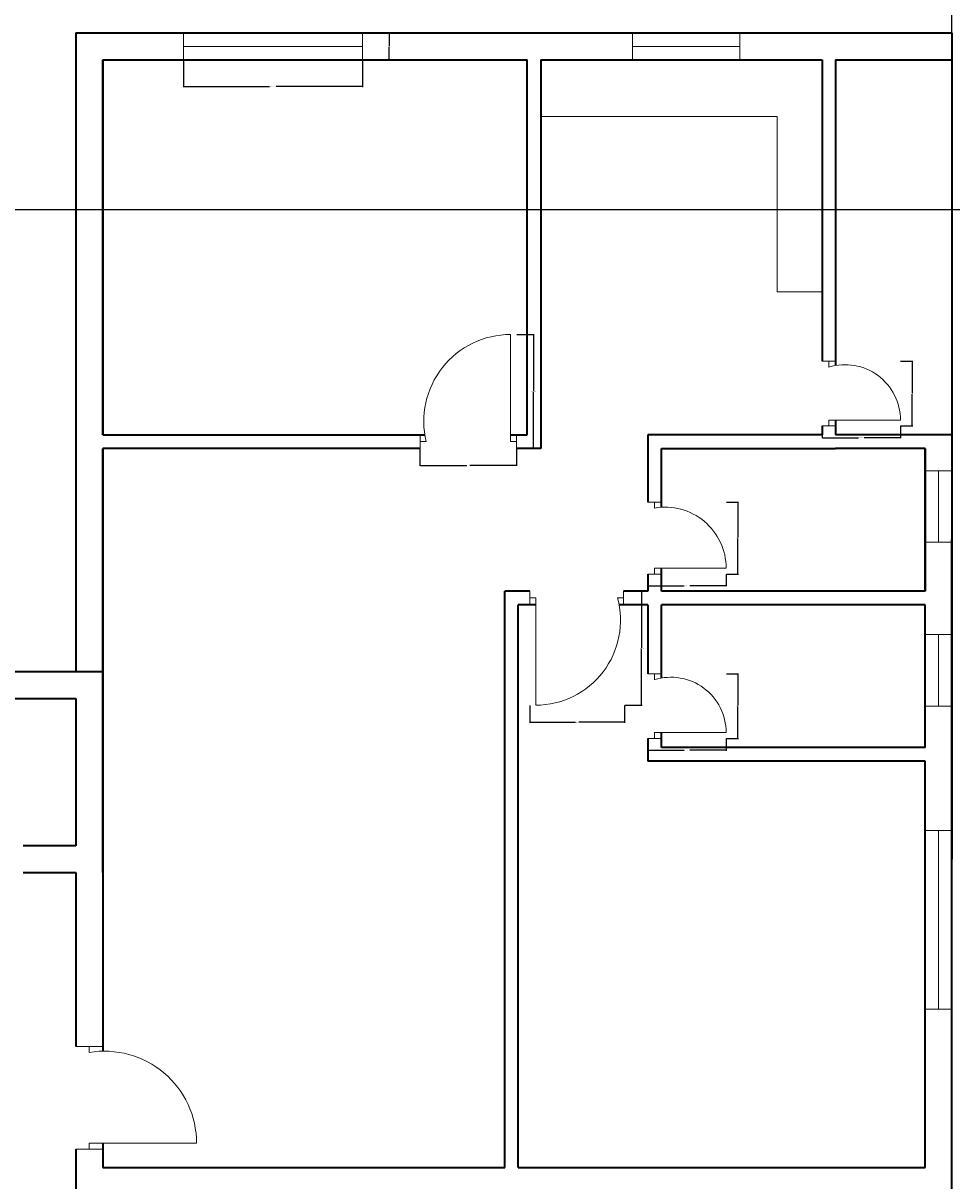
# Model space of a CAD drawing. Units: inches. Extents: x 2120 to 4013, y 1390 to 3019.
# Tile 53 of 59: x 3507 to 3819, y 1967 to 2356. Entities that reach past the tile are written whole.
import ezdxf

# ---------------------------------------------------------------- set-up
doc = ezdxf.new("R2010")
doc.units = ezdxf.units.IN
for name, color, linetype, lineweight in [('A-ANNO-DIMS', 2, 'Continuous', 18), ('A-ANNO-SYMB', 2, 'Continuous', 25), ('A-DOOR', 3, 'Continuous', 18), ('A-FLOR-CASE', 8, 'Continuous', 18), ('A-FURN', 8, 'Continuous', 13), ('A-GLAZ', 4, 'Continuous', 18), ('A-WALL', 7, 'Continuous', 35)]:
    doc.layers.add(name, color=color, linetype=linetype, lineweight=lineweight)
doc.styles.get("Standard").update_dxf_attribs({"font": 'arial.ttf'})
doc.dimstyles.get("Standard").update_dxf_attribs({"dimtxt": 0.18, "dimasz": 0.18, "dimexe": 0.18, "dimexo": 0.0625, "dimgap": 0.09, "dimtad": 0, "dimtih": 1, "dimtoh": 1, "dimdec": 4, "dimzin": 0, "dimdsep": 46, "dimtxsty": 'Standard', "dimcen": 0.09, "dimadec": 0, "dimazin": 0, "dimtfac": 1, "dimtdec": 4, "dimtofl": 0, "dimtmove": 0, "dimatfit": 3, "dimfxl": 1, "dimtolj": 1, "dimtzin": 0, "dimarcsym": 0})

# ---------------------------------------------------------------- blocks, each defined once
blk = doc.blocks.new('DOOR-SWING-24IN-106p92DEG')
for p, q in [((4.5, 21.79), (0, 21.79)), ((0, 21.79), (2.25, 21.79)), ((2.25, 21.79), (2.25, 19.79)), ((2.25, 0), (2.25, 2)), ((2.25, 2), (26.25, 2)), ((0, 0), (4.5, 0)), ((4.5, 0), (2.25, 0))]:
    blk.add_line(p, q)
blk.add_arc((7.66, 2), 18.59, 0, 106.9181)
blk = doc.blocks.new('DOOR-SWING-24IN-99p98DEG')
for p, q in [((0, 24.15), (4.5, 24.15)), ((4.5, 24.15), (2.25, 24.15)), ((2.25, 24.15), (2.25, 22.15)), ((4.5, 0), (0, 0)), ((0, 0), (2.25, 0)), ((2.25, 0), (2.25, 2)), ((2.25, 2), (26.25, 2))]:
    blk.add_line(p, q)
blk.add_arc((5.79, 2), 20.46, 0, 99.9792)
blk = doc.blocks.new('DOOR-SWING-24IN-107p06DEG')
for p, q in [((0, 21.74), (4.5, 21.74)), ((4.5, 21.74), (2.25, 21.74)), ((2.25, 21.74), (2.25, 19.74)), ((4.5, 0), (0, 0)), ((0, 0), (0, 0)), ((0, 0), (2.25, 0)), ((2.25, 0), (2.25, 2)), ((2.25, 2), (26.25, 2))]:
    blk.add_line(p, q)
blk.add_arc((7.69, 2), 18.56, 0, 107.0611)
blk = doc.blocks.new('DOOR-SWING-36IN-103p63DEG')
for p, q in [((30.32, 2.25), (30.32, 38.25)), ((0, 4.5), (0, 0)), ((32.32, 4.5), (32.32, 0)), ((0, 0), (0, 2.25)), ((0, 2.25), (2, 2.25)), ((32.32, 2.25), (30.32, 2.25)), ((32.32, 0), (32.32, 2.25))]:
    blk.add_line(p, q)
blk.add_arc((30.32, 9.11), 29.14, 90, 193.6269)
blk = doc.blocks.new('DOOR-SWING-36IN-105p32DEG')
for p, q in [((0, 33.75), (0, 38.25)), ((0, 38.25), (0, 36)), ((0, 36), (2, 36)), ((2, 36), (2, 0)), ((31.46, 36), (29.46, 36)), ((31.46, 33.75), (31.46, 38.25)), ((31.46, 38.25), (31.46, 36))]:
    blk.add_line(p, q)
blk.add_arc((2, 28.48), 28.48, 270, 15.3194)
blk = doc.blocks.new('WIN-PLAN-24IN-02')
for p, q in [((0, 0), (0, 9)), ((0, 9), (0, 4.5)), ((24, 4.5), (24, 9)), ((24, 9), (24, 0)), ((0, 4.5), (24, 4.5))]:
    blk.add_line(p, q)
blk = doc.blocks.new('WIN-PLAN-24IN-04')
for p, q in [((0, 24), (9, 24)), ((9, 24), (4.5, 24)), ((4.5, 24), (4.5, 0)), ((9, 24), (9, 24)), ((4.5, 0), (0, 0)), ((0, 0), (9, 0))]:
    blk.add_line(p, q)
blk = doc.blocks.new('WIN-PLAN-60IN')
for p, q in [((0, 9), (0, 0)), ((60, 4.5), (60, 9)), ((60, 9), (60, 0)), ((0, 0), (0, 4.5)), ((0, 4.5), (60, 4.5))]:
    blk.add_line(p, q)
blk = doc.blocks.new('WIN-PLAN-60IN-02')
for p, q in [((0, 0), (0, 9)), ((0, 9), (0, 4.5)), ((60, 4.5), (60, 9)), ((60, 9), (60, 0)), ((0, 4.5), (60, 4.5))]:
    blk.add_line(p, q)
blk = doc.blocks.new('WIN-PLAN-36IN')
for p, q in [((0, 0), (0, 9)), ((0, 9), (0, 4.5)), ((36, 4.5), (36, 9)), ((36, 9), (36, 0)), ((0, 4.5), (36, 4.5))]:
    blk.add_line(p, q)
blk = doc.blocks.new('*D121')
at = {"layer": 'A-ANNO-DIMS', "color": 0, "lineweight": -2, "transparency": 16777216}
for p, q in [((3775.23, 2220.48), (3775.23, 2216.43)), ((3801.48, 2220.48), (3801.48, 2216.43)), ((3775.41, 2216.61), (3787.37, 2216.61)), ((3801.3, 2216.61), (3789.35, 2216.61))]:
    blk.add_line(p, q, dxfattribs=at)
at = {"layer": 'A-ANNO-DIMS', "color": 0, "transparency": 16777216}
for points in [[(3775.41, 2216.64), (3775.41, 2216.58), (3775.23, 2216.61)], [(3801.3, 2216.64), (3801.3, 2216.58), (3801.48, 2216.61)]]:
    blk.add_solid(points, dxfattribs=at)
at = {"layer": 'Defpoints', "color": 0, "transparency": 16777216}
for p in [(3775.23, 2220.54), (3801.48, 2220.54), (3801.48, 2216.61)]:
    blk.add_point(p, dxfattribs=at)
at = {"layer": 'A-ANNO-DIMS', "color": 0, "transparency": 16777216, "insert": (3788.36, 2216.61), "char_height": 0.18, "attachment_point": 5}
blk.add_mtext('\\A1;SWING 26 TYP.', dxfattribs=at)
blk = doc.blocks.new('*D122')
at = {"layer": 'A-ANNO-DIMS', "color": 0, "lineweight": -2, "transparency": 16777216}
for p, q in [((3801.55, 2242.33), (3805.6, 2242.33)), ((3805.42, 2242.15), (3805.42, 2231.62)), ((3805.42, 2220.72), (3805.42, 2231.25)), ((3801.55, 2220.54), (3805.6, 2220.54))]:
    blk.add_line(p, q, dxfattribs=at)
at = {"layer": 'A-ANNO-DIMS', "color": 0, "transparency": 16777216}
for points in [[(3805.39, 2242.15), (3805.45, 2242.15), (3805.42, 2242.33)], [(3805.39, 2220.72), (3805.45, 2220.72), (3805.42, 2220.54)]]:
    blk.add_solid(points, dxfattribs=at)
at = {"layer": 'Defpoints', "color": 0, "transparency": 16777216}
for p in [(3801.48, 2242.33), (3805.42, 2242.33), (3801.48, 2220.54)]:
    blk.add_point(p, dxfattribs=at)
at = {"layer": 'A-ANNO-DIMS', "color": 0, "transparency": 16777216, "insert": (3805.42, 2231.44), "char_height": 0.18, "attachment_point": 5}
blk.add_mtext('\\A1;22 TYP.', dxfattribs=at)
blk = doc.blocks.new('*D123')
at = {"layer": 'A-ANNO-DIMS', "color": 0, "lineweight": -2, "transparency": 16777216}
for p, q in [((3716.73, 2170.76), (3716.73, 2166.7)), ((3742.98, 2170.76), (3742.98, 2166.7)), ((3716.91, 2166.88), (3728.87, 2166.88)), ((3742.8, 2166.88), (3730.85, 2166.88))]:
    blk.add_line(p, q, dxfattribs=at)
at = {"layer": 'A-ANNO-DIMS', "color": 0, "transparency": 16777216}
for points in [[(3716.91, 2166.91), (3716.91, 2166.85), (3716.73, 2166.88)], [(3742.8, 2166.91), (3742.8, 2166.85), (3742.98, 2166.88)]]:
    blk.add_solid(points, dxfattribs=at)
at = {"layer": 'Defpoints', "color": 0, "transparency": 16777216}
for p in [(3716.73, 2170.82), (3742.98, 2170.82), (3742.98, 2166.88)]:
    blk.add_point(p, dxfattribs=at)
at = {"layer": 'A-ANNO-DIMS', "color": 0, "transparency": 16777216, "insert": (3729.86, 2166.88), "char_height": 0.18, "attachment_point": 5}
blk.add_mtext('\\A1;SWING 26 TYP.', dxfattribs=at)
blk = doc.blocks.new('*D124')
at = {"layer": 'A-ANNO-DIMS', "color": 0, "lineweight": -2, "transparency": 16777216}
for p, q in [((3743.05, 2194.97), (3747.1, 2194.97)), ((3746.92, 2194.79), (3746.92, 2183.07)), ((3746.92, 2171), (3746.92, 2182.71)), ((3743.05, 2170.82), (3747.1, 2170.82))]:
    blk.add_line(p, q, dxfattribs=at)
at = {"layer": 'A-ANNO-DIMS', "color": 0, "transparency": 16777216}
for points in [[(3746.89, 2194.79), (3746.95, 2194.79), (3746.92, 2194.97)], [(3746.89, 2171), (3746.95, 2171), (3746.92, 2170.82)]]:
    blk.add_solid(points, dxfattribs=at)
at = {"layer": 'Defpoints', "color": 0, "transparency": 16777216}
for p in [(3742.98, 2194.97), (3746.92, 2194.97), (3742.98, 2170.82)]:
    blk.add_point(p, dxfattribs=at)
at = {"layer": 'A-ANNO-DIMS', "color": 0, "transparency": 16777216, "insert": (3746.92, 2182.89), "char_height": 0.18, "attachment_point": 5}
blk.add_mtext('\\A1;24 TYP.', dxfattribs=at)
blk = doc.blocks.new('*D125')
at = {"layer": 'A-ANNO-DIMS', "color": 0, "lineweight": -2, "transparency": 16777216}
for p, q in [((3716.73, 2115.54), (3716.73, 2111.49)), ((3742.98, 2115.54), (3742.98, 2111.49)), ((3716.91, 2111.67), (3728.87, 2111.67)), ((3742.8, 2111.67), (3730.85, 2111.67))]:
    blk.add_line(p, q, dxfattribs=at)
at = {"layer": 'A-ANNO-DIMS', "color": 0, "transparency": 16777216}
for points in [[(3716.91, 2111.7), (3716.91, 2111.64), (3716.73, 2111.67)], [(3742.8, 2111.7), (3742.8, 2111.64), (3742.98, 2111.67)]]:
    blk.add_solid(points, dxfattribs=at)
at = {"layer": 'Defpoints', "color": 0, "transparency": 16777216}
for p in [(3716.73, 2115.6), (3742.98, 2115.6), (3742.98, 2111.67)]:
    blk.add_point(p, dxfattribs=at)
at = {"layer": 'A-ANNO-DIMS', "color": 0, "transparency": 16777216, "insert": (3729.86, 2111.67), "char_height": 0.18, "attachment_point": 5}
blk.add_mtext('\\A1;SWING 26 TYP.', dxfattribs=at)
blk = doc.blocks.new('*D126')
at = {"layer": 'A-ANNO-DIMS', "color": 0, "lineweight": -2, "transparency": 16777216}
for p, q in [((3743.05, 2137.34), (3747.1, 2137.34)), ((3746.92, 2137.16), (3746.92, 2126.65)), ((3746.92, 2115.78), (3746.92, 2126.29)), ((3743.05, 2115.6), (3747.1, 2115.6))]:
    blk.add_line(p, q, dxfattribs=at)
at = {"layer": 'A-ANNO-DIMS', "color": 0, "transparency": 16777216}
for points in [[(3746.89, 2137.16), (3746.95, 2137.16), (3746.92, 2137.34)], [(3746.89, 2115.78), (3746.95, 2115.78), (3746.92, 2115.6)]]:
    blk.add_solid(points, dxfattribs=at)
at = {"layer": 'Defpoints', "color": 0, "transparency": 16777216}
for p in [(3742.98, 2137.34), (3746.92, 2137.34), (3742.98, 2115.6)]:
    blk.add_point(p, dxfattribs=at)
at = {"layer": 'A-ANNO-DIMS', "color": 0, "transparency": 16777216, "insert": (3746.92, 2126.47), "char_height": 0.18, "attachment_point": 5}
blk.add_mtext('\\A1;22 TYP.', dxfattribs=at)
blk = doc.blocks.new('*D151')
at = {"layer": 'A-ANNO-DIMS', "color": 0, "lineweight": -2, "transparency": 16777216}
for p, q in [((3672.7, 2251.28), (3678.56, 2251.28)), ((3678.38, 2251.1), (3678.38, 2232.34)), ((3678.38, 2213.21), (3678.38, 2231.97)), ((3672.7, 2213.03), (3678.56, 2213.03))]:
    blk.add_line(p, q, dxfattribs=at)
at = {"layer": 'A-ANNO-DIMS', "color": 0, "transparency": 16777216}
for points in [[(3678.35, 2251.1), (3678.41, 2251.1), (3678.38, 2251.28)], [(3678.35, 2213.21), (3678.41, 2213.21), (3678.38, 2213.03)]]:
    blk.add_solid(points, dxfattribs=at)
at = {"layer": 'Defpoints', "color": 0, "transparency": 16777216}
for p in [(3672.64, 2251.28), (3678.38, 2251.28), (3672.64, 2213.03)]:
    blk.add_point(p, dxfattribs=at)
at = {"layer": 'A-ANNO-DIMS', "color": 0, "transparency": 16777216, "insert": (3678.38, 2232.16), "char_height": 0.18, "attachment_point": 5}
blk.add_mtext('\\A1;SWING 38 TYP.', dxfattribs=at)
blk = doc.blocks.new('*D152')
at = {"layer": 'A-ANNO-DIMS', "color": 0, "lineweight": -2, "transparency": 16777216}
for p, q in [((3640.22, 2212.97), (3640.22, 2207.11)), ((3672.64, 2212.97), (3672.64, 2207.11)), ((3640.4, 2207.29), (3655.9, 2207.29)), ((3672.46, 2207.29), (3656.96, 2207.29))]:
    blk.add_line(p, q, dxfattribs=at)
at = {"layer": 'A-ANNO-DIMS', "color": 0, "transparency": 16777216}
for points in [[(3640.4, 2207.32), (3640.4, 2207.26), (3640.22, 2207.29)], [(3672.46, 2207.32), (3672.46, 2207.26), (3672.64, 2207.29)]]:
    blk.add_solid(points, dxfattribs=at)
at = {"layer": 'Defpoints', "color": 0, "transparency": 16777216}
for p in [(3640.22, 2213.03), (3672.64, 2213.03), (3672.64, 2207.29)]:
    blk.add_point(p, dxfattribs=at)
at = {"layer": 'A-ANNO-DIMS', "color": 0, "transparency": 16777216, "insert": (3656.43, 2207.29), "char_height": 0.18, "attachment_point": 5}
blk.add_mtext('\\A1;32 TYP.', dxfattribs=at)
blk = doc.blocks.new('*D153')
at = {"layer": 'A-ANNO-DIMS', "color": 0, "lineweight": -2, "transparency": 16777216}
for p, q in [((3708.93, 2165.03), (3714.78, 2165.03)), ((3714.6, 2164.85), (3714.6, 2146.09)), ((3714.6, 2126.96), (3714.6, 2145.72)), ((3708.93, 2126.78), (3714.78, 2126.78))]:
    blk.add_line(p, q, dxfattribs=at)
at = {"layer": 'A-ANNO-DIMS', "color": 0, "transparency": 16777216}
for points in [[(3714.57, 2164.85), (3714.63, 2164.85), (3714.6, 2165.03)], [(3714.57, 2126.96), (3714.63, 2126.96), (3714.6, 2126.78)]]:
    blk.add_solid(points, dxfattribs=at)
at = {"layer": 'Defpoints', "color": 0, "transparency": 16777216}
for p in [(3708.86, 2165.03), (3714.6, 2165.03), (3708.86, 2126.78)]:
    blk.add_point(p, dxfattribs=at)
at = {"layer": 'A-ANNO-DIMS', "color": 0, "transparency": 16777216, "insert": (3714.6, 2145.91), "char_height": 0.18, "attachment_point": 5}
blk.add_mtext('\\A1;SWING 38 TYP.', dxfattribs=at)
blk = doc.blocks.new('*D154')
at = {"layer": 'A-ANNO-DIMS', "color": 0, "lineweight": -2, "transparency": 16777216}
for p, q in [((3677.05, 2126.72), (3677.05, 2120.86)), ((3708.86, 2126.72), (3708.86, 2120.86)), ((3677.23, 2121.04), (3692.43, 2121.04)), ((3708.68, 2121.04), (3693.49, 2121.04))]:
    blk.add_line(p, q, dxfattribs=at)
at = {"layer": 'A-ANNO-DIMS', "color": 0, "transparency": 16777216}
for points in [[(3677.23, 2121.07), (3677.23, 2121.01), (3677.05, 2121.04)], [(3708.68, 2121.07), (3708.68, 2121.01), (3708.86, 2121.04)]]:
    blk.add_solid(points, dxfattribs=at)
at = {"layer": 'Defpoints', "color": 0, "transparency": 16777216}
for p in [(3677.05, 2126.78), (3708.86, 2126.78), (3708.86, 2121.04)]:
    blk.add_point(p, dxfattribs=at)
at = {"layer": 'A-ANNO-DIMS', "color": 0, "transparency": 16777216, "insert": (3692.96, 2121.04), "char_height": 0.18, "attachment_point": 5}
blk.add_mtext('\\A1;32 TYP.', dxfattribs=at)
blk = doc.blocks.new('*D173')
at = {"layer": 'A-ANNO-DIMS', "color": 0, "lineweight": -2, "transparency": 16777216}
for p, q in [((3560.88, 2343.47), (3560.88, 2334.35)), ((3620.88, 2343.47), (3620.88, 2334.35)), ((3561.06, 2334.53), (3589.76, 2334.53)), ((3620.7, 2334.53), (3592, 2334.53))]:
    blk.add_line(p, q, dxfattribs=at)
at = {"layer": 'A-ANNO-DIMS', "color": 0, "transparency": 16777216}
for points in [[(3561.06, 2334.56), (3561.06, 2334.5), (3560.88, 2334.53)], [(3620.7, 2334.56), (3620.7, 2334.5), (3620.88, 2334.53)]]:
    blk.add_solid(points, dxfattribs=at)
at = {"layer": 'Defpoints', "color": 0, "transparency": 16777216}
for p in [(3560.88, 2343.53), (3620.88, 2343.53), (3620.88, 2334.53)]:
    blk.add_point(p, dxfattribs=at)
at = {"layer": 'A-ANNO-DIMS', "color": 0, "transparency": 16777216, "insert": (3590.88, 2334.53), "char_height": 0.18, "attachment_point": 5}
blk.add_mtext('\\A1;WINDOW 60 TYP.', dxfattribs=at)
blk = doc.blocks.new('*D174')
at = {"layer": 'A-ANNO-DIMS', "color": 0, "lineweight": -2, "transparency": 16777216}
for p, q in [((3620.94, 2352.53), (3630.06, 2352.53)), ((3629.88, 2352.35), (3629.88, 2348.21)), ((3629.88, 2343.71), (3629.88, 2347.85)), ((3620.94, 2343.53), (3630.06, 2343.53))]:
    blk.add_line(p, q, dxfattribs=at)
at = {"layer": 'A-ANNO-DIMS', "color": 0, "transparency": 16777216}
for points in [[(3629.85, 2352.35), (3629.91, 2352.35), (3629.88, 2352.53)], [(3629.85, 2343.71), (3629.91, 2343.71), (3629.88, 2343.53)]]:
    blk.add_solid(points, dxfattribs=at)
at = {"layer": 'Defpoints', "color": 0, "transparency": 16777216}
for p in [(3620.88, 2352.53), (3629.88, 2352.53), (3620.88, 2343.53)]:
    blk.add_point(p, dxfattribs=at)
at = {"layer": 'A-ANNO-DIMS', "color": 0, "transparency": 16777216, "insert": (3629.88, 2348.03), "char_height": 0.18, "attachment_point": 5}
blk.add_mtext('\\A1;9 TYP.', dxfattribs=at)
blk = doc.blocks.new('*D216')
at = {"layer": 'A-ANNO-DIMS', "color": 0, "lineweight": -2, "transparency": 16777216}
for p, q in [((3071.73, 2352.59), (3071.73, 2396.46)), ((3071.91, 2396.28), (3444.95, 2396.28)), ((3818.55, 2396.28), (3445.52, 2396.28)), ((3818.73, 2352.59), (3818.73, 2396.46))]:
    blk.add_line(p, q, dxfattribs=at)
at = {"layer": 'A-ANNO-DIMS', "color": 0, "transparency": 16777216}
for points in [[(3071.91, 2396.31), (3071.91, 2396.25), (3071.73, 2396.28)], [(3818.55, 2396.31), (3818.55, 2396.25), (3818.73, 2396.28)]]:
    blk.add_solid(points, dxfattribs=at)
at = {"layer": 'Defpoints', "color": 0, "transparency": 16777216}
for p in [(3818.73, 2396.28), (3071.73, 2352.53), (3818.73, 2352.53)]:
    blk.add_point(p, dxfattribs=at)
at = {"layer": 'A-ANNO-DIMS', "color": 0, "transparency": 16777216, "insert": (3445.23, 2396.28), "char_height": 0.18, "attachment_point": 5}
blk.add_mtext('\\A1;747', dxfattribs=at)

msp = doc.modelspace()

# ---------------------------------------------------------------- linework, layer by layer
at = {"layer": 'A-ANNO-SYMB'}
msp.add_line((3024.2377, 2293.2324), (3883.8033, 2293.2324), dxfattribs=at)
at = {"layer": 'A-DOOR'}
for p, q in [((3533.7347, 2012.1531), (3524.7347, 2012.1531)), ((3529.2347, 2012.1531), (3529.2347, 2010.1531)), ((3529.2347, 1977.7015), (3529.2347, 1979.7015)), ((3529.2347, 1979.7015), (3565.2347, 1979.7015)), ((3533.7347, 1977.7015), (3524.7347, 1977.7015)), ((3524.7347, 1977.7015), (3529.2347, 1977.7015))]:
    msp.add_line(p, q, dxfattribs=at)
msp.add_arc((3534.3555, 1979.7015), 30.8792, 360, 99.545687, dxfattribs=at)
at = {"layer": 'A-FLOR-CASE'}
for p, q in [((3680.7347, 2324.4835), (3760.0811, 2324.4835)), ((3760.0811, 2324.4835), (3760.0811, 2265.6008)), ((3760.0811, 2265.6008), (3775.2347, 2265.6008))]:
    msp.add_line(p, q, dxfattribs=at)
at = {"layer": 'A-FURN'}
for p, q in [((3558.231, 2343.531), (3606.0213, 2343.531)), ((3809.7347, 2054.2058), (3809.7347, 2006.4156))]:
    msp.add_line(p, q, dxfattribs=at)
at = {"layer": 'A-WALL'}
for p, q in [((3524.7347, 2352.531), (3818.7347, 2352.531)), ((3524.7347, 2352.531), (3524.7347, 2138.031)), ((3818.7347, 2352.531), (3818.7347, 2075.031)), ((3533.7347, 2343.531), (3676.2347, 2343.531)), ((3533.7347, 2217.531), (3533.7347, 2343.531)), ((3533.7347, 2343.531), (3533.7347, 2217.531)), ((3676.2347, 2217.531), (3676.2347, 2343.531)), ((3680.7347, 2343.531), (3775.2347, 2343.531)), ((3680.7347, 2343.531), (3680.7347, 2217.531)), ((3775.2347, 2343.531), (3775.2347, 2242.3281)), ((3779.7347, 2343.531), (3818.7347, 2343.531)), ((3779.7347, 2343.531), (3779.7347, 2240.8622)), ((3779.7347, 2343.531), (3818.7347, 2343.531)), ((3775.2347, 2220.5425), (3775.2347, 2217.531)), ((3779.7347, 2222.5425), (3779.7347, 2217.531)), ((3533.7347, 2217.531), (3641.87, 2217.531)), ((3670.6379, 2217.531), (3676.2347, 2217.531)), ((3680.7347, 2217.531), (3680.7347, 2213.031)), ((3720.7767, 2217.531), (3716.7347, 2217.531)), ((3716.7347, 2217.531), (3716.7347, 2213.031)), ((3775.2347, 2217.531), (3720.7767, 2217.531)), ((3818.7347, 2217.531), (3779.7347, 2217.531)), ((3533.7347, 2138.031), (3533.7347, 2213.031)), ((3640.3224, 2213.031), (3533.7347, 2213.031)), ((3533.7347, 2213.031), (3533.7347, 2010.5745)), ((3680.7347, 2213.031), (3672.6379, 2213.031)), ((3716.7347, 2213.031), (3716.7347, 2194.9663)), ((3721.2347, 2213.031), (3779.7347, 2213.031)), ((3721.2347, 2193.2348), (3721.2347, 2213.031)), ((3809.7347, 2213.031), (3779.7347, 2213.031)), ((3809.7347, 2182.408), (3809.7347, 2213.031)), ((3809.7347, 2213.031), (3809.7347, 2165.031)), ((3809.7347, 2165.031), (3809.7347, 2182.408)), ((3818.7347, 1971.531), (3818.7347, 2182.408)), ((3716.7347, 2170.8205), (3716.7347, 2165.031)), ((3721.2347, 2165.031), (3721.2347, 2172.8205)), ((3668.7347, 1971.531), (3668.7347, 2165.031)), ((3677.0538, 2165.031), (3668.7347, 2165.031)), ((3716.7347, 2165.031), (3708.5184, 2165.031)), ((3809.7347, 2165.031), (3721.2347, 2165.031)), ((3673.2347, 1971.531), (3673.2347, 2160.531)), ((3679.0538, 2160.531), (3673.2347, 2160.531)), ((3716.7347, 2160.531), (3707.0377, 2160.531)), ((3716.7347, 2160.531), (3716.7347, 2137.3432)), ((3809.7347, 2160.531), (3721.2347, 2160.531)), ((3721.2347, 2135.8828), (3721.2347, 2160.531)), ((3809.7347, 2112.531), (3809.7347, 2160.531)), ((3533.7347, 2138.031), (3437.7347, 2138.031)), ((3533.7347, 2129.031), (3533.7347, 2138.031)), ((3446.7347, 2129.031), (3524.7347, 2129.031)), ((3524.7347, 2129.031), (3524.7347, 2079.531)), ((3533.7347, 2070.531), (3533.7347, 2129.031)), ((3716.7347, 2115.6039), (3716.7347, 2108.031)), ((3721.2347, 2112.531), (3721.2347, 2117.6039)), ((3809.7347, 2112.531), (3721.2347, 2112.531)), ((3809.7347, 2108.031), (3716.7347, 2108.031)), ((3809.7347, 1971.531), (3809.7347, 2108.031)), ((3524.7347, 2079.531), (3507.0394, 2079.531)), ((3533.7347, 2070.531), (3533.7347, 2079.531)), ((3507.0394, 2070.531), (3524.7347, 2070.531)), ((3524.7347, 2070.531), (3524.7347, 2012.1531)), ((3533.7347, 1979.7015), (3533.7347, 1971.531)), ((3524.7347, 1977.7015), (3524.7347, 1962.531)), ((3533.7347, 1971.531), (3668.7347, 1971.531)), ((3673.2347, 1971.531), (3809.7347, 1971.531)), ((3818.7347, 1962.531), (3818.7347, 1971.531))]:
    msp.add_line(p, q, dxfattribs=at)

# ---------------------------------------------------------------- block references
at = {"layer": 'A-DOOR'}
for name, p in [('DOOR-SWING-36IN-103p63DEG', (3640.3224, 2213.031)), ('DOOR-SWING-24IN-106p92DEG', (3775.2347, 2220.5425)), ('DOOR-SWING-24IN-99p98DEG', (3716.7347, 2170.8205)), ('DOOR-SWING-36IN-105p32DEG', (3677.0538, 2126.781)), ('DOOR-SWING-24IN-107p06DEG', (3716.7347, 2115.6039))]:
    msp.add_blockref(name, p, dxfattribs=at)
at = {"layer": 'A-GLAZ'}
for name, p in [('WIN-PLAN-60IN-02', (3560.877, 2343.531)), ('WIN-PLAN-36IN', (3711.5315, 2343.531)), ('WIN-PLAN-24IN-04', (3809.7347, 2181.523))]:
    msp.add_blockref(name, p, dxfattribs=at)
for name, p, rotation in [('WIN-PLAN-24IN-02', (3809.7347, 2150.4993), 269.9999999999982), ('WIN-PLAN-60IN', (3809.7347, 2084.7256), 269.9999999999992)]:
    msp.add_blockref(name, p, dxfattribs=dict(at, rotation=rotation))

# ---------------------------------------------------------------- dimensions: what is measured, and where the dimension line sits
at = {"layer": 'A-ANNO-DIMS'}
dim = msp.add_linear_dim(base=(3818.7347, 2396.281), p1=(3071.7347, 2352.531), p2=(3818.7347, 2352.531), dimstyle='Standard', override={"dimdec": 0, "dimlfac": 1, "dimrnd": 0, "dimzin": 0, "dimdsep": 46, "dimlunit": 2}, dxfattribs=at)
dim.commit()
dim.dimension.update_dxf_attribs({"geometry": '*D216', "text_midpoint": (3445.2347, 2396.281)})
for base, p1, p2, text, picture, middle in [((3629.877, 2352.531), (3620.877, 2343.531), (3620.877, 2352.531), '<> TYP.', '*D174', (3629.877, 2348.031)), ((3678.3754, 2251.281), (3672.6379, 2213.031), (3672.6379, 2251.281), 'SWING <> TYP.', '*D151', (3678.3754, 2232.156)), ((3805.4222, 2242.3281), (3801.4847, 2220.5425), (3801.4847, 2242.3281), '<> TYP.', '*D122', (3805.4222, 2231.4353)), ((3746.9222, 2194.9663), (3742.9847, 2170.8205), (3742.9847, 2194.9663), '<> TYP.', '*D124', (3746.9222, 2182.8934)), ((3714.6023, 2165.031), (3708.8648, 2126.781), (3708.8648, 2165.031), 'SWING <> TYP.', '*D153', (3714.6023, 2145.906)), ((3746.9222, 2137.3432), (3742.9847, 2115.6039), (3742.9847, 2137.3432), '<> TYP.', '*D126', (3746.9222, 2126.4735))]:
    dim = msp.add_linear_dim(base=base, p1=p1, p2=p2, angle=90, text=text, dimstyle='Standard', override={"dimdec": 0, "dimlfac": 1, "dimrnd": 0, "dimzin": 0, "dimdsep": 46, "dimlunit": 2}, dxfattribs=at)
    dim.commit()
    dim.dimension.update_dxf_attribs({"geometry": picture, "text_midpoint": middle})
for base, p1, p2, text, picture, middle in [((3620.877, 2334.531), (3560.877, 2343.531), (3620.877, 2343.531), 'WINDOW <> TYP.', '*D173', (3590.877, 2334.531)), ((3801.4847, 2216.605), (3775.2347, 2220.5425), (3801.4847, 2220.5425), 'SWING <> TYP.', '*D121', (3788.3597, 2216.605)), ((3672.6379, 2207.2935), (3640.2172, 2213.031), (3672.6379, 2213.031), '<> TYP.', '*D152', (3656.4276, 2207.2935)), ((3742.9847, 2166.883), (3716.7347, 2170.8205), (3742.9847, 2170.8205), 'SWING <> TYP.', '*D123', (3729.8597, 2166.883)), ((3708.8648, 2121.0435), (3677.0538, 2126.781), (3708.8648, 2126.781), '<> TYP.', '*D154', (3692.9593, 2121.0435)), ((3742.9847, 2111.6664), (3716.7347, 2115.6039), (3742.9847, 2115.6039), 'SWING <> TYP.', '*D125', (3729.8597, 2111.6664))]:
    dim = msp.add_linear_dim(base=base, p1=p1, p2=p2, text=text, dimstyle='Standard', override={"dimdec": 0, "dimlfac": 1, "dimrnd": 0, "dimzin": 0, "dimdsep": 46, "dimlunit": 2}, dxfattribs=at)
    dim.commit()
    dim.dimension.update_dxf_attribs({"geometry": picture, "text_midpoint": middle})

doc.saveas('drawing.dxf')
